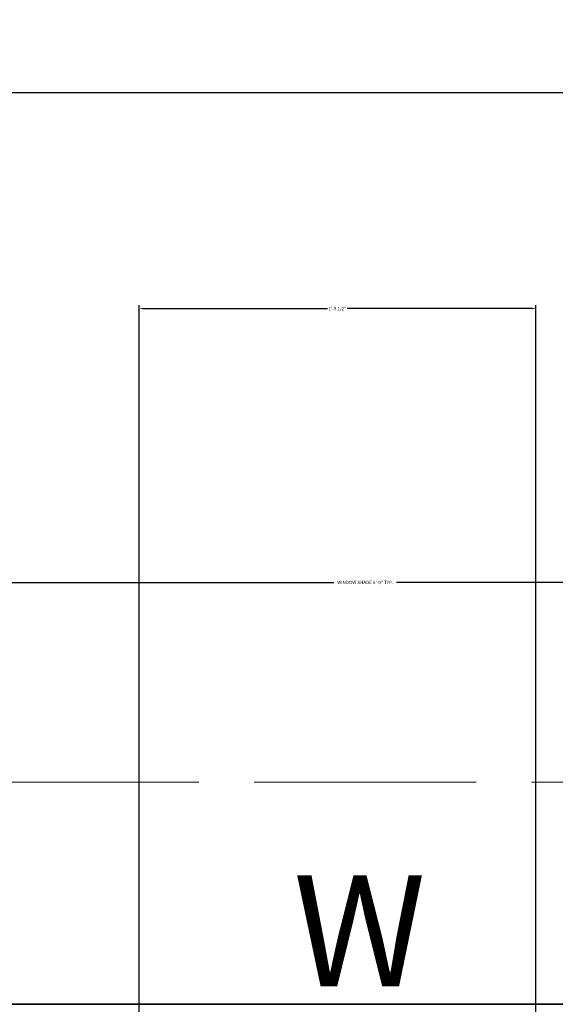
# Model space of a CAD drawing. Units: inches. Extents: x -5 to 482, y -460 to 66.
# Tile 28 of 31: x 77 to 106, y 13 to 66. Entities that reach past the tile are written whole.
import ezdxf

# ---------------------------------------------------------------- set-up
doc = ezdxf.new("R2010")
doc.units = ezdxf.units.IN
doc.header["$MEASUREMENT"] = 0
doc.linetypes.add('ACAD_ISO02W100', pattern=[15, 12, -3])
for name, color, linetype, lineweight in [('A-ANNO-DIMS', 2, 'Continuous', 18), ('A-ANNO-TEXT', 7, 'Continuous', 18), ('A-GLAZ-OVHD', 4, 'ACAD_ISO02W100', 13), ('A-WALL', 7, 'Continuous', 35)]:
    doc.layers.add(name, color=color, linetype=linetype, lineweight=lineweight)
doc.styles.get("Standard").update_dxf_attribs({"font": 'arial.ttf'})
doc.dimstyles.get("Standard").update_dxf_attribs({"dimtxt": 0.18, "dimasz": 0.18, "dimexe": 0.18, "dimexo": 0.0625, "dimgap": 0.09, "dimtad": 0, "dimtih": 1, "dimtoh": 1, "dimdec": 0, "dimzin": 0, "dimdsep": 46, "dimlunit": 3, "dimtxsty": 'Standard', "dimcen": 0.09, "dimadec": 0, "dimazin": 0, "dimtfac": 1, "dimtdec": 0, "dimtofl": 0, "dimtmove": 0, "dimatfit": 3, "dimfxl": 1, "dimtolj": 1, "dimtzin": 0, "dimarcsym": 0})

# ---------------------------------------------------------------- blocks, each defined once
blk = doc.blocks.new('*D3')
at = {"layer": 'A-ANNO-DIMS', "color": 0, "lineweight": -2, "transparency": 16777216}
for p, q in [((32.877, 13.214), (32.877, 62.612)), ((33.057, 62.432), (221.233, 62.432)), ((430.197, 62.432), (242.02, 62.432)), ((430.377, 13.214), (430.377, 62.612))]:
    blk.add_line(p, q, dxfattribs=at)
at = {"layer": 'A-ANNO-DIMS', "color": 0, "transparency": 16777216}
for points in [[(33.057, 62.462), (33.057, 62.402), (32.877, 62.432)], [(430.197, 62.462), (430.197, 62.402), (430.377, 62.432)]]:
    blk.add_solid(points, dxfattribs=at)
at = {"layer": 'Defpoints', "color": 0, "transparency": 16777216}
for p in [(430.377, 62.432), (32.877, 13.151), (430.377, 13.151)]:
    blk.add_point(p, dxfattribs=at)
at = {"layer": 'A-ANNO-DIMS', "color": 0, "transparency": 16777216, "insert": (231.627, 62.432), "char_height": 6, "attachment_point": 5}
blk.add_mtext('\\A1;33\'-2"', dxfattribs=at)
blk = doc.blocks.new('WIN-SHADE-72IN')
blk.add_line((0, 12), (72, 12))
blk = doc.blocks.new('*D45')
at = {"layer": 'A-ANNO-DIMS', "color": 0, "lineweight": -2, "transparency": 16777216}
for p, q in [((59.948, 25.214), (59.948, 36.131)), ((60.128, 35.951), (94.251, 35.951)), ((131.768, 35.951), (97.645, 35.951)), ((131.948, 25.214), (131.948, 36.131))]:
    blk.add_line(p, q, dxfattribs=at)
at = {"layer": 'A-ANNO-DIMS', "color": 0, "transparency": 16777216}
for points in [[(60.128, 35.981), (60.128, 35.921), (59.948, 35.951)], [(131.768, 35.981), (131.768, 35.921), (131.948, 35.951)]]:
    blk.add_solid(points, dxfattribs=at)
at = {"layer": 'Defpoints', "color": 0, "transparency": 16777216}
for p in [(131.948, 35.951), (59.948, 25.151), (131.948, 25.151)]:
    blk.add_point(p, dxfattribs=at)
at = {"layer": 'A-ANNO-DIMS', "color": 0, "transparency": 16777216, "insert": (95.948, 35.951), "char_height": 0.18, "attachment_point": 5}
blk.add_mtext('\\A1;WINDOW SHADE 6\'-0" TYP.', dxfattribs=at)
blk = doc.blocks.new('*D69')
at = {"layer": 'A-ANNO-DIMS', "color": 0, "lineweight": -2, "transparency": 16777216}
for p, q in [((83.715, 2.351), (83.715, 50.931)), ((83.895, 50.751), (93.912, 50.751)), ((104.991, 50.751), (94.973, 50.751)), ((105.171, 2.351), (105.171, 50.931))]:
    blk.add_line(p, q, dxfattribs=at)
at = {"layer": 'A-ANNO-DIMS', "color": 0, "transparency": 16777216}
for points in [[(83.895, 50.781), (83.895, 50.721), (83.715, 50.751)], [(104.991, 50.781), (104.991, 50.721), (105.171, 50.751)]]:
    blk.add_solid(points, dxfattribs=at)
at = {"layer": 'Defpoints', "color": 0, "transparency": 16777216}
for p in [(105.171, 50.751), (83.715, 2.288), (105.171, 2.288)]:
    blk.add_point(p, dxfattribs=at)
at = {"layer": 'A-ANNO-DIMS', "color": 0, "transparency": 16777216, "insert": (94.443, 50.751), "char_height": 0.18, "attachment_point": 5}
blk.add_mtext('\\A1;1\'-9 1/2"', dxfattribs=at)

msp = doc.modelspace()

# ---------------------------------------------------------------- linework, layer by layer
at = {"layer": 'A-WALL'}
msp.add_line((32.877, 13.151), (430.377, 13.151), dxfattribs=at)

# ---------------------------------------------------------------- block references
at = {"layer": 'A-GLAZ-OVHD'}
msp.add_blockref('WIN-SHADE-72IN', (59.948, 13.151), dxfattribs=at)

# ---------------------------------------------------------------- texts
at = {"layer": 'A-ANNO-TEXT', "insert": (92.05, 20.129), "char_height": 6, "attachment_point": 1}
msp.add_mtext('W', dxfattribs=at)

# ---------------------------------------------------------------- dimensions: what is measured, and where the dimension line sits
at = {"layer": 'A-ANNO-DIMS'}
for base, p1, p2, override, picture, middle in [((430.376735986, 62.431571932), (32.876735986, 13.151335974), (430.376735986, 13.151335974), {"dimtxt": 6, "dimclrd": 0, "dimclre": 0, "dimclrt": 0}, '*D3', (231.626735986, 62.431571932)), ((105.171, 50.751), (83.715, 2.288), (105.171, 2.288), {"dimdec": 1, "dimlfac": 1, "dimrnd": 0, "dimzin": 1, "dimdsep": 46, "dimlunit": 4, "dimfrac": 2}, '*D69', (94.443, 50.751))]:
    dim = msp.add_linear_dim(base=base, p1=p1, p2=p2, dimstyle='Standard', override=override, dxfattribs=at)
    dim.commit()
    dim.dimension.update_dxf_attribs({"geometry": picture, "text_midpoint": middle})
dim = msp.add_linear_dim(base=(131.948, 35.951), p1=(59.948, 25.151), p2=(131.948, 25.151), text='WINDOW SHADE <> TYP.', dimstyle='Standard', override={"dimdec": 1, "dimlfac": 1, "dimrnd": 0, "dimzin": 1, "dimdsep": 46, "dimlunit": 4, "dimfrac": 2}, dxfattribs=at)
dim.commit()
dim.dimension.update_dxf_attribs({"geometry": '*D45', "text_midpoint": (95.948, 35.951)})

doc.saveas('drawing.dxf')
